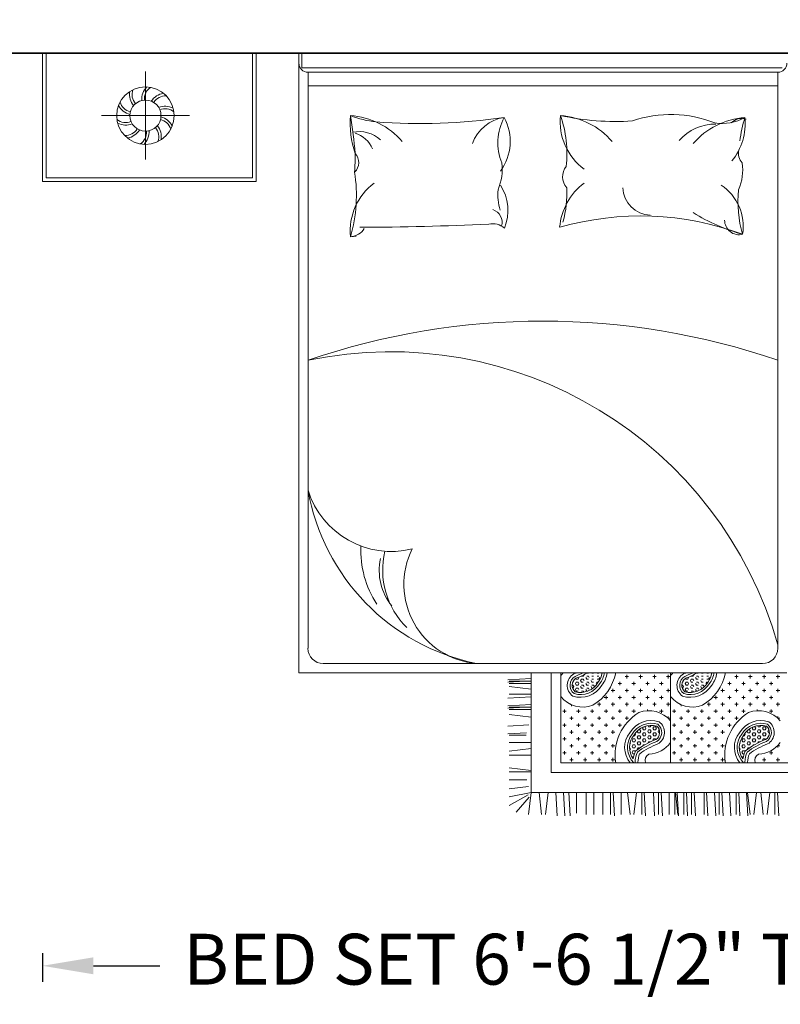
# Model space of a CAD drawing. Units: inches. Extents: x -638 to 186, y -762 to 59.
# Tile 23 of 31: x -125 to -66, y -126 to -48. Entities that reach past the tile are written whole.
import ezdxf

# ---------------------------------------------------------------- set-up
doc = ezdxf.new("R2010")
doc.units = ezdxf.units.IN
for name, color, linetype, lineweight in [('A-ANNO-DIMS', 2, 'Continuous', 18), ('furn', 8, 'Continuous', 13), ('wall', 7, 'Continuous', 35)]:
    doc.layers.add(name, color=color, linetype=linetype, lineweight=lineweight)
doc.styles.get("Standard").update_dxf_attribs({"font": 'arial.ttf'})
doc.dimstyles.new('ISO-25', dxfattribs={"dimtxt": 4, "dimasz": 4, "dimexe": 1.25, "dimexo": 0.625, "dimtad": 0, "dimlunit": 4, "dimtxsty": 'Standard', "dimcen": 2.5, "dimclrt": 256, "dimadec": 0, "dimazin": 0, "dimtfac": 1, "dimtmove": 0, "dimatfit": 3, "dimfxl": 1, "dimfxlon": 1, "dimarcsym": 0})

# ---------------------------------------------------------------- blocks, each defined once
blk = doc.blocks.new('BED-DOUBLE-WITH-NIGHTSTANDS')
for p, q in [((0, 59.951), (78.699, 59.951)), ((0, 49.874), (0, 59.951)), ((0.288, 50.162), (0.288, 59.951)), ((16.508, 59.951), (16.508, 50.162)), ((16.796, 59.951), (16.796, 49.874)), ((20.158, 59.951), (20.158, 11.244)), ((20.398, 58.826), (20.398, 59.951)), ((8.091, 51.596), (8.091, 58.516)), ((58.161, 58.826), (20.398, 58.826)), ((20.878, 58.468), (57.828, 58.468)), ((20.878, 58.468), (20.878, 13.164)), ((57.828, 13.164), (57.828, 58.468)), ((57.828, 57.404), (20.878, 57.404)), ((4.631, 55.056), (11.551, 55.056)), ((16.796, 49.874), (0, 49.874)), ((16.508, 50.162), (0.288, 50.162)), ((22.077, 11.964), (56.628, 11.964)), ((20.158, 11.244), (58.548, 11.244)), ((38.435, 1.829), (38.435, 11.244)), ((39.99, 3.384), (39.99, 11.244)), ((40.767, 4.161), (40.767, 11.244)), ((42.184, 10.861), (42.116, 10.743)), ((42.164, 10.895), (42.184, 10.861)), ((42.381, 10.99), (42.388, 10.979)), ((42.524, 10.979), (42.388, 10.979)), ((42.588, 11.09), (42.524, 10.979)), ((42.728, 10.861), (42.796, 10.743)), ((42.932, 10.979), (42.796, 10.979)), ((42.932, 11.215), (42.819, 11.215)), ((42.932, 10.979), (43, 10.861)), ((43.34, 11.215), (43.204, 11.215)), ((43.34, 10.979), (43.204, 10.979)), ((43.748, 11.215), (43.612, 11.215)), ((43.748, 10.979), (43.612, 10.979)), ((43.816, 10.861), (43.748, 10.743)), ((44.002, 11.184), (43.952, 11.097)), ((45.812, 10.936), (46.084, 10.936)), ((45.948, 10.8), (45.948, 11.072)), ((46.9, 10.936), (47.172, 10.936)), ((47.036, 10.8), (47.036, 11.072)), ((47.989, 10.936), (48.261, 10.936)), ((48.125, 10.8), (48.125, 11.072)), ((49.077, 10.936), (49.349, 10.936)), ((49.213, 10.8), (49.213, 11.072)), ((49.395, 11.244), (49.395, 4.161)), ((50.811, 10.861), (50.743, 10.743)), ((50.792, 10.895), (50.811, 10.861)), ((51.009, 10.99), (51.015, 10.979)), ((51.151, 10.979), (51.015, 10.979)), ((51.216, 11.09), (51.151, 10.979)), ((51.355, 10.861), (51.424, 10.743)), ((51.56, 10.979), (51.424, 10.979)), ((51.56, 11.215), (51.447, 11.215)), ((51.56, 10.979), (51.628, 10.861)), ((51.968, 11.215), (51.832, 11.215)), ((51.968, 10.979), (51.832, 10.979)), ((52.376, 11.215), (52.24, 11.215)), ((52.376, 10.979), (52.24, 10.979)), ((52.444, 10.861), (52.376, 10.743)), ((52.63, 11.184), (52.58, 11.097)), ((54.44, 10.936), (54.712, 10.936)), ((54.576, 10.8), (54.576, 11.072)), ((55.528, 10.936), (55.8, 10.936)), ((55.664, 10.8), (55.664, 11.072)), ((56.616, 10.936), (56.888, 10.936)), ((56.752, 10.8), (56.752, 11.072)), ((57.705, 10.936), (57.977, 10.936)), ((57.841, 10.8), (57.841, 11.072)), ((38.435, 10.789), (36.606, 10.687)), ((38.435, 10.606), (36.606, 10.504)), ((38.435, 10.585), (36.707, 10.585)), ((38.435, 10.402), (36.707, 10.402)), ((38.435, 9.957), (36.707, 10.161)), ((41.708, 10.272), (41.649, 10.272)), ((41.708, 10.508), (41.699, 10.508)), ((41.776, 10.625), (41.708, 10.508)), ((41.708, 10.272), (41.776, 10.154)), ((41.776, 10.154), (41.708, 10.036)), ((41.77, 10.636), (41.776, 10.625)), ((41.98, 10.508), (41.912, 10.39)), ((41.912, 10.39), (41.98, 10.272)), ((41.943, 10.806), (41.98, 10.743)), ((42.116, 10.743), (41.98, 10.743)), ((42.116, 10.508), (41.98, 10.508)), ((42.116, 10.272), (41.98, 10.272)), ((42.116, 10.508), (42.184, 10.39)), ((42.184, 10.39), (42.116, 10.272)), ((42.388, 10.743), (42.32, 10.625)), ((42.32, 10.625), (42.388, 10.508)), ((42.32, 10.154), (42.388, 10.036)), ((42.524, 10.743), (42.388, 10.743)), ((42.524, 10.508), (42.388, 10.508)), ((42.524, 10.272), (42.388, 10.272)), ((42.524, 10.743), (42.592, 10.625)), ((42.524, 10.272), (42.592, 10.154)), ((42.728, 10.39), (42.796, 10.272)), ((42.932, 10.743), (42.796, 10.743)), ((42.932, 10.508), (42.796, 10.508)), ((42.932, 10.272), (42.796, 10.272)), ((42.932, 10.508), (43, 10.39)), ((43.136, 10.625), (43.204, 10.508)), ((43.136, 10.154), (43.204, 10.036)), ((43.34, 10.743), (43.204, 10.743)), ((43.34, 10.508), (43.204, 10.508)), ((43.34, 10.272), (43.204, 10.272)), ((43.34, 10.272), (43.408, 10.154)), ((43.408, 10.154), (43.381, 10.108)), ((43.612, 10.508), (43.544, 10.39)), ((43.748, 10.743), (43.612, 10.743)), ((43.703, 10.508), (43.612, 10.508)), ((45.268, 10.392), (45.54, 10.392)), ((45.404, 10.256), (45.404, 10.528)), ((46.356, 10.392), (46.628, 10.392)), ((46.492, 10.256), (46.492, 10.528)), ((47.445, 10.392), (47.717, 10.392)), ((47.581, 10.256), (47.581, 10.528)), ((48.533, 10.392), (48.805, 10.392)), ((48.669, 10.256), (48.669, 10.528)), ((50.335, 10.272), (50.277, 10.272)), ((50.335, 10.508), (50.327, 10.508)), ((50.403, 10.625), (50.335, 10.508)), ((50.335, 10.272), (50.403, 10.154)), ((50.403, 10.154), (50.335, 10.036)), ((50.397, 10.636), (50.403, 10.625)), ((50.607, 10.508), (50.539, 10.39)), ((50.539, 10.39), (50.607, 10.272)), ((50.571, 10.806), (50.607, 10.743)), ((50.743, 10.743), (50.607, 10.743)), ((50.743, 10.508), (50.607, 10.508)), ((50.743, 10.272), (50.607, 10.272)), ((50.743, 10.508), (50.811, 10.39)), ((50.811, 10.39), (50.743, 10.272)), ((51.015, 10.743), (50.947, 10.625)), ((50.947, 10.625), (51.015, 10.508)), ((50.947, 10.154), (51.015, 10.036)), ((51.151, 10.743), (51.015, 10.743)), ((51.151, 10.508), (51.015, 10.508)), ((51.151, 10.272), (51.015, 10.272)), ((51.151, 10.743), (51.219, 10.625)), ((51.151, 10.272), (51.219, 10.154)), ((51.355, 10.39), (51.424, 10.272)), ((51.56, 10.743), (51.424, 10.743)), ((51.56, 10.508), (51.424, 10.508)), ((51.56, 10.272), (51.424, 10.272)), ((51.56, 10.508), (51.628, 10.39)), ((51.764, 10.625), (51.832, 10.508)), ((51.764, 10.154), (51.832, 10.036)), ((51.968, 10.743), (51.832, 10.743)), ((51.968, 10.508), (51.832, 10.508)), ((51.968, 10.272), (51.832, 10.272)), ((51.968, 10.272), (52.036, 10.154)), ((52.036, 10.154), (52.009, 10.108)), ((52.24, 10.508), (52.172, 10.39)), ((52.376, 10.743), (52.24, 10.743)), ((52.33, 10.508), (52.24, 10.508)), ((53.896, 10.392), (54.168, 10.392)), ((54.032, 10.256), (54.032, 10.528)), ((54.984, 10.392), (55.256, 10.392)), ((55.12, 10.256), (55.12, 10.528)), ((56.072, 10.392), (56.344, 10.392)), ((56.208, 10.256), (56.208, 10.528)), ((57.161, 10.392), (57.433, 10.392)), ((57.297, 10.256), (57.297, 10.528)), ((38.435, 9.347), (36.606, 9.245)), ((38.435, 9.55), (36.707, 9.55)), ((41.708, 10.036), (41.685, 10.036)), ((41.98, 10.036), (41.912, 9.919)), ((41.912, 9.919), (41.98, 9.801)), ((42.116, 10.036), (41.98, 10.036)), ((42.116, 9.801), (41.98, 9.801)), ((42.116, 10.036), (42.184, 9.919)), ((42.524, 10.036), (42.388, 10.036)), ((42.524, 9.801), (42.388, 9.801)), ((42.524, 9.801), (42.574, 9.713)), ((42.728, 9.919), (42.796, 9.801)), ((42.932, 10.036), (42.796, 10.036)), ((42.888, 9.801), (42.796, 9.801)), ((42.932, 10.036), (43, 9.919)), ((43.297, 10.036), (43.204, 10.036)), ((44.18, 9.303), (44.452, 9.303)), ((44.316, 9.167), (44.316, 9.439)), ((44.724, 9.847), (44.996, 9.847)), ((44.86, 9.711), (44.86, 9.983)), ((45.268, 9.303), (45.54, 9.303)), ((45.404, 9.167), (45.404, 9.439)), ((45.812, 9.847), (46.084, 9.847)), ((45.948, 9.711), (45.948, 9.983)), ((46.356, 9.303), (46.628, 9.303)), ((46.492, 9.167), (46.492, 9.439)), ((46.9, 9.847), (47.172, 9.847)), ((47.036, 9.711), (47.036, 9.983)), ((47.445, 9.303), (47.717, 9.303)), ((47.581, 9.167), (47.581, 9.439)), ((47.989, 9.847), (48.261, 9.847)), ((48.125, 9.711), (48.125, 9.983)), ((48.533, 9.303), (48.805, 9.303)), ((48.669, 9.167), (48.669, 9.439)), ((49.077, 9.847), (49.349, 9.847)), ((49.213, 9.711), (49.213, 9.983)), ((50.335, 10.036), (50.313, 10.036)), ((50.607, 10.036), (50.539, 9.919)), ((50.539, 9.919), (50.607, 9.801)), ((50.743, 10.036), (50.607, 10.036)), ((50.743, 9.801), (50.607, 9.801)), ((50.743, 10.036), (50.811, 9.919)), ((51.151, 10.036), (51.015, 10.036)), ((51.151, 9.801), (51.015, 9.801)), ((51.151, 9.801), (51.202, 9.713)), ((51.355, 9.919), (51.424, 9.801)), ((51.56, 10.036), (51.424, 10.036)), ((51.516, 9.801), (51.424, 9.801)), ((51.56, 10.036), (51.628, 9.919)), ((51.925, 10.036), (51.832, 10.036)), ((52.807, 9.303), (53.079, 9.303)), ((52.943, 9.167), (52.943, 9.439)), ((53.351, 9.847), (53.623, 9.847)), ((53.487, 9.711), (53.487, 9.983)), ((53.896, 9.303), (54.168, 9.303)), ((54.032, 9.167), (54.032, 9.439)), ((54.44, 9.847), (54.712, 9.847)), ((54.576, 9.711), (54.576, 9.983)), ((54.984, 9.303), (55.256, 9.303)), ((55.12, 9.167), (55.12, 9.439)), ((55.528, 9.847), (55.8, 9.847)), ((55.664, 9.711), (55.664, 9.983)), ((56.072, 9.303), (56.344, 9.303)), ((56.208, 9.167), (56.208, 9.439)), ((56.616, 9.847), (56.888, 9.847)), ((56.752, 9.711), (56.752, 9.983)), ((57.161, 9.303), (57.433, 9.303)), ((57.297, 9.167), (57.297, 9.439)), ((57.705, 9.847), (57.977, 9.847)), ((57.841, 9.711), (57.841, 9.983)), ((38.435, 8.736), (36.606, 8.634)), ((38.435, 8.553), (36.606, 8.451)), ((38.435, 8.532), (36.707, 8.532)), ((41.459, 8.759), (41.528, 8.759)), ((41.595, 8.623), (41.595, 8.728)), ((43.635, 8.759), (43.907, 8.759)), ((43.771, 8.623), (43.771, 8.895)), ((44.724, 8.759), (44.996, 8.759)), ((44.86, 8.623), (44.86, 8.895)), ((45.812, 8.759), (46.084, 8.759)), ((45.948, 8.623), (45.948, 8.895)), ((46.9, 8.759), (47.172, 8.759)), ((47.036, 8.623), (47.036, 8.895)), ((47.989, 8.759), (48.261, 8.759)), ((48.125, 8.623), (48.125, 8.895)), ((49.077, 8.759), (49.349, 8.759)), ((49.213, 8.623), (49.213, 8.895)), ((50.086, 8.759), (50.155, 8.759)), ((50.222, 8.623), (50.222, 8.728)), ((52.263, 8.759), (52.535, 8.759)), ((52.399, 8.623), (52.399, 8.895)), ((53.351, 8.759), (53.623, 8.759)), ((53.487, 8.623), (53.487, 8.895)), ((54.44, 8.759), (54.712, 8.759)), ((54.576, 8.623), (54.576, 8.895)), ((55.528, 8.759), (55.8, 8.759)), ((55.664, 8.623), (55.664, 8.895)), ((56.616, 8.759), (56.888, 8.759)), ((56.752, 8.623), (56.752, 8.895)), ((57.705, 8.759), (57.977, 8.759)), ((57.841, 8.623), (57.841, 8.895)), ((38.435, 8.349), (36.707, 8.349)), ((38.435, 7.757), (36.707, 7.961)), ((40.914, 8.215), (41.187, 8.215)), ((41.051, 8.079), (41.051, 8.351)), ((41.595, 7.535), (41.595, 7.807)), ((42.003, 8.215), (42.275, 8.215)), ((42.139, 8.079), (42.139, 8.351)), ((42.683, 7.535), (42.683, 7.807)), ((43.091, 8.215), (43.363, 8.215)), ((43.227, 8.079), (43.227, 8.351)), ((43.771, 7.535), (43.771, 7.807)), ((44.18, 8.215), (44.452, 8.215)), ((44.316, 8.079), (44.316, 8.351)), ((44.86, 7.535), (44.86, 7.807)), ((45.268, 8.215), (45.54, 8.215)), ((45.404, 8.079), (45.404, 8.351)), ((45.948, 7.535), (45.948, 7.807)), ((46.356, 8.215), (46.628, 8.215)), ((46.492, 8.079), (46.492, 8.351)), ((47.581, 8.253), (47.581, 8.351)), ((48.533, 8.215), (48.805, 8.215)), ((48.669, 8.079), (48.669, 8.351)), ((49.213, 7.653), (49.213, 7.807)), ((49.542, 8.215), (49.814, 8.215)), ((49.678, 8.079), (49.678, 8.351)), ((50.222, 7.535), (50.222, 7.807)), ((50.63, 8.215), (50.903, 8.215)), ((50.767, 8.079), (50.767, 8.351)), ((51.311, 7.535), (51.311, 7.807)), ((51.719, 8.215), (51.991, 8.215)), ((51.855, 8.079), (51.855, 8.351)), ((52.399, 7.535), (52.399, 7.807)), ((52.807, 8.215), (53.079, 8.215)), ((52.943, 8.079), (52.943, 8.351)), ((53.487, 7.535), (53.487, 7.807)), ((53.896, 8.215), (54.168, 8.215)), ((54.032, 8.079), (54.032, 8.351)), ((54.576, 7.535), (54.576, 7.807)), ((54.984, 8.215), (55.256, 8.215)), ((55.12, 8.079), (55.12, 8.351)), ((56.208, 8.253), (56.208, 8.351)), ((57.161, 8.215), (57.433, 8.215)), ((57.297, 8.079), (57.297, 8.351)), ((57.841, 7.653), (57.841, 7.807)), ((38.233, 7.135), (36.606, 7.044)), ((40.914, 7.127), (41.187, 7.127)), ((41.051, 6.99), (41.051, 7.263)), ((41.459, 7.671), (41.731, 7.671)), ((42.003, 7.127), (42.275, 7.127)), ((42.139, 6.99), (42.139, 7.263)), ((42.547, 7.671), (42.819, 7.671)), ((43.091, 7.127), (43.363, 7.127)), ((43.227, 6.99), (43.227, 7.263)), ((43.635, 7.671), (43.907, 7.671)), ((44.18, 7.127), (44.452, 7.127)), ((44.316, 6.99), (44.316, 7.263)), ((44.724, 7.671), (44.996, 7.671)), ((45.268, 7.127), (45.54, 7.127)), ((45.404, 6.99), (45.404, 7.263)), ((45.812, 7.671), (46.084, 7.671)), ((47.185, 6.877), (47.239, 6.971)), ((47.297, 6.995), (47.389, 6.995)), ((47.457, 6.877), (47.389, 6.995)), ((47.661, 6.995), (47.611, 7.082)), ((47.661, 6.995), (47.797, 6.995)), ((47.797, 6.995), (47.861, 7.105)), ((48.001, 6.877), (48.069, 6.995)), ((48.069, 6.995), (48.205, 6.995)), ((48.273, 6.877), (48.205, 6.995)), ((49.195, 7.671), (49.349, 7.671)), ((49.542, 7.127), (49.814, 7.127)), ((49.678, 6.99), (49.678, 7.263)), ((50.086, 7.671), (50.358, 7.671)), ((50.63, 7.127), (50.903, 7.127)), ((50.767, 6.99), (50.767, 7.263)), ((51.175, 7.671), (51.447, 7.671)), ((51.719, 7.127), (51.991, 7.127)), ((51.855, 6.99), (51.855, 7.263)), ((52.263, 7.671), (52.535, 7.671)), ((52.807, 7.127), (53.079, 7.127)), ((52.943, 6.99), (52.943, 7.263)), ((53.351, 7.671), (53.623, 7.671)), ((53.896, 7.127), (54.168, 7.127)), ((54.032, 6.99), (54.032, 7.263)), ((54.44, 7.671), (54.712, 7.671)), ((55.813, 6.877), (55.867, 6.971)), ((55.924, 6.995), (56.017, 6.995)), ((56.085, 6.877), (56.017, 6.995)), ((56.289, 6.995), (56.238, 7.082)), ((56.289, 6.995), (56.425, 6.995)), ((56.425, 6.995), (56.488, 7.105)), ((56.629, 6.877), (56.697, 6.995)), ((56.697, 6.995), (56.833, 6.995)), ((56.901, 6.877), (56.833, 6.995)), ((57.822, 7.671), (57.977, 7.671)), ((38.06, 6.514), (36.606, 6.433)), ((38.024, 6.332), (36.707, 6.332)), ((41.459, 6.582), (41.731, 6.582)), ((41.595, 6.446), (41.595, 6.718)), ((42.547, 6.582), (42.819, 6.582)), ((42.683, 6.446), (42.683, 6.718)), ((43.635, 6.582), (43.907, 6.582)), ((43.771, 6.446), (43.771, 6.718)), ((44.724, 6.582), (44.996, 6.582)), ((44.86, 6.446), (44.86, 6.718)), ((46.482, 6.288), (46.573, 6.288)), ((46.573, 6.288), (46.641, 6.406)), ((46.641, 6.406), (46.605, 6.469)), ((46.777, 6.642), (46.803, 6.688)), ((46.845, 6.524), (46.777, 6.642)), ((46.777, 6.17), (46.845, 6.288)), ((46.845, 6.524), (46.981, 6.524)), ((46.845, 6.288), (46.981, 6.288)), ((46.888, 6.76), (46.981, 6.76)), ((47.049, 6.642), (46.981, 6.76)), ((46.981, 6.524), (47.049, 6.642)), ((47.049, 6.17), (46.981, 6.288)), ((47.253, 6.76), (47.185, 6.877)), ((47.185, 6.406), (47.253, 6.524)), ((47.253, 6.288), (47.185, 6.406)), ((47.253, 6.76), (47.389, 6.76)), ((47.253, 6.524), (47.389, 6.524)), ((47.253, 6.288), (47.389, 6.288)), ((47.389, 6.76), (47.457, 6.877)), ((47.457, 6.406), (47.389, 6.524)), ((47.389, 6.288), (47.457, 6.406)), ((47.593, 6.642), (47.661, 6.76)), ((47.661, 6.524), (47.593, 6.642)), ((47.593, 6.17), (47.661, 6.288)), ((47.661, 6.76), (47.797, 6.76)), ((47.661, 6.524), (47.797, 6.524)), ((47.661, 6.288), (47.797, 6.288)), ((47.865, 6.642), (47.797, 6.76)), ((47.797, 6.524), (47.865, 6.642)), ((47.865, 6.17), (47.797, 6.288)), ((48.069, 6.76), (48.001, 6.877)), ((48.001, 6.406), (48.069, 6.524)), ((48.069, 6.288), (48.001, 6.406)), ((48.069, 6.76), (48.205, 6.76)), ((48.069, 6.524), (48.205, 6.524)), ((48.069, 6.288), (48.205, 6.288)), ((48.205, 6.76), (48.273, 6.877)), ((48.273, 6.406), (48.205, 6.524)), ((48.205, 6.288), (48.273, 6.406)), ((48.409, 6.642), (48.477, 6.76)), ((48.477, 6.524), (48.409, 6.642)), ((48.409, 6.17), (48.477, 6.288)), ((48.477, 6.76), (48.5, 6.76)), ((48.477, 6.524), (48.536, 6.524)), ((48.477, 6.288), (48.486, 6.288)), ((50.086, 6.582), (50.358, 6.582)), ((50.222, 6.446), (50.222, 6.718)), ((51.175, 6.582), (51.447, 6.582)), ((51.311, 6.446), (51.311, 6.718)), ((52.263, 6.582), (52.535, 6.582)), ((52.399, 6.446), (52.399, 6.718)), ((53.351, 6.582), (53.623, 6.582)), ((53.487, 6.446), (53.487, 6.718)), ((55.11, 6.288), (55.201, 6.288)), ((55.201, 6.288), (55.269, 6.406)), ((55.269, 6.406), (55.232, 6.469)), ((55.405, 6.642), (55.431, 6.688)), ((55.473, 6.524), (55.405, 6.642)), ((55.405, 6.17), (55.473, 6.288)), ((55.473, 6.524), (55.609, 6.524)), ((55.473, 6.288), (55.609, 6.288)), ((55.515, 6.76), (55.609, 6.76)), ((55.677, 6.642), (55.609, 6.76)), ((55.609, 6.524), (55.677, 6.642)), ((55.677, 6.17), (55.609, 6.288)), ((55.881, 6.76), (55.813, 6.877)), ((55.813, 6.406), (55.881, 6.524)), ((55.881, 6.288), (55.813, 6.406)), ((55.881, 6.76), (56.017, 6.76)), ((55.881, 6.524), (56.017, 6.524)), ((55.881, 6.288), (56.017, 6.288)), ((56.017, 6.76), (56.085, 6.877)), ((56.085, 6.406), (56.017, 6.524)), ((56.017, 6.288), (56.085, 6.406)), ((56.221, 6.642), (56.289, 6.76)), ((56.289, 6.524), (56.221, 6.642)), ((56.221, 6.17), (56.289, 6.288)), ((56.289, 6.76), (56.425, 6.76)), ((56.289, 6.524), (56.425, 6.524)), ((56.289, 6.288), (56.425, 6.288)), ((56.493, 6.642), (56.425, 6.76)), ((56.425, 6.524), (56.493, 6.642)), ((56.493, 6.17), (56.425, 6.288)), ((56.697, 6.76), (56.629, 6.877)), ((56.629, 6.406), (56.697, 6.524)), ((56.697, 6.288), (56.629, 6.406)), ((56.697, 6.76), (56.833, 6.76)), ((56.697, 6.524), (56.833, 6.524)), ((56.697, 6.288), (56.833, 6.288)), ((56.833, 6.76), (56.901, 6.877)), ((56.901, 6.406), (56.833, 6.524)), ((56.833, 6.288), (56.901, 6.406)), ((57.037, 6.642), (57.105, 6.76)), ((57.105, 6.524), (57.037, 6.642)), ((57.037, 6.17), (57.105, 6.288)), ((57.105, 6.76), (57.128, 6.76)), ((57.105, 6.524), (57.164, 6.524)), ((57.105, 6.288), (57.113, 6.288)), ((38.435, 5.764), (36.71, 5.764)), ((40.914, 6.038), (41.187, 6.038)), ((41.051, 5.902), (41.051, 6.174)), ((41.459, 5.494), (41.731, 5.494)), ((41.595, 5.358), (41.595, 5.63)), ((42.003, 6.038), (42.275, 6.038)), ((42.139, 5.902), (42.139, 6.174)), ((42.547, 5.494), (42.819, 5.494)), ((42.683, 5.358), (42.683, 5.63)), ((43.091, 6.038), (43.363, 6.038)), ((43.227, 5.902), (43.227, 6.174)), ((43.635, 5.494), (43.907, 5.494)), ((43.771, 5.358), (43.771, 5.63)), ((44.18, 6.038), (44.452, 6.038)), ((44.316, 5.902), (44.316, 6.174)), ((44.724, 5.494), (44.996, 5.494)), ((44.86, 5.358), (44.86, 5.63)), ((46.183, 5.612), (46.233, 5.699)), ((46.233, 5.699), (46.21, 5.739)), ((46.369, 5.935), (46.437, 6.053)), ((46.437, 5.817), (46.369, 5.935)), ((46.369, 5.464), (46.437, 5.581)), ((46.437, 5.346), (46.369, 5.464)), ((46.437, 6.053), (46.573, 6.053)), ((46.437, 5.817), (46.573, 5.817)), ((46.437, 5.581), (46.573, 5.581)), ((46.641, 5.935), (46.573, 6.053)), ((46.573, 5.817), (46.641, 5.935)), ((46.641, 5.464), (46.573, 5.581)), ((46.573, 5.346), (46.641, 5.464)), ((46.845, 6.053), (46.777, 6.17)), ((46.777, 5.699), (46.845, 5.817)), ((46.845, 5.581), (46.777, 5.699)), ((46.845, 6.053), (46.981, 6.053)), ((46.845, 5.817), (46.981, 5.817)), ((46.845, 5.581), (46.981, 5.581)), ((46.981, 6.053), (47.049, 6.17)), ((47.049, 5.699), (46.981, 5.817)), ((46.981, 5.581), (47.049, 5.699)), ((47.185, 5.935), (47.253, 6.053)), ((47.253, 5.817), (47.185, 5.935)), ((47.195, 5.481), (47.253, 5.581)), ((47.253, 6.053), (47.389, 6.053)), ((47.253, 5.817), (47.389, 5.817)), ((47.253, 5.581), (47.365, 5.581)), ((47.457, 5.935), (47.389, 6.053)), ((47.389, 5.817), (47.457, 5.935)), ((47.661, 6.053), (47.593, 6.17)), ((47.597, 5.706), (47.661, 5.817)), ((47.661, 6.053), (47.797, 6.053)), ((47.661, 5.817), (47.797, 5.817)), ((47.797, 6.053), (47.865, 6.17)), ((47.804, 5.806), (47.797, 5.817)), ((48.001, 5.935), (48.069, 6.053)), ((48.021, 5.901), (48.001, 5.935)), ((48.069, 6.053), (48.205, 6.053)), ((48.242, 5.99), (48.205, 6.053)), ((48.415, 6.16), (48.409, 6.17)), ((49.542, 6.038), (49.814, 6.038)), ((49.678, 5.902), (49.678, 6.174)), ((50.086, 5.494), (50.358, 5.494)), ((50.222, 5.358), (50.222, 5.63)), ((50.63, 6.038), (50.903, 6.038)), ((50.767, 5.902), (50.767, 6.174)), ((51.175, 5.494), (51.447, 5.494)), ((51.311, 5.358), (51.311, 5.63)), ((51.719, 6.038), (51.991, 6.038)), ((51.855, 5.902), (51.855, 6.174)), ((52.263, 5.494), (52.535, 5.494)), ((52.399, 5.358), (52.399, 5.63)), ((52.807, 6.038), (53.079, 6.038)), ((52.943, 5.902), (52.943, 6.174)), ((53.351, 5.494), (53.623, 5.494)), ((53.487, 5.358), (53.487, 5.63)), ((54.81, 5.612), (54.86, 5.699)), ((54.86, 5.699), (54.837, 5.739)), ((54.996, 5.935), (55.064, 6.053)), ((55.064, 5.817), (54.996, 5.935)), ((54.996, 5.464), (55.064, 5.581)), ((55.064, 5.346), (54.996, 5.464)), ((55.064, 6.053), (55.201, 6.053)), ((55.064, 5.817), (55.201, 5.817)), ((55.064, 5.581), (55.201, 5.581)), ((55.269, 5.935), (55.201, 6.053)), ((55.201, 5.817), (55.269, 5.935)), ((55.269, 5.464), (55.201, 5.581)), ((55.201, 5.346), (55.269, 5.464)), ((55.473, 6.053), (55.405, 6.17)), ((55.405, 5.699), (55.473, 5.817)), ((55.473, 5.581), (55.405, 5.699)), ((55.473, 6.053), (55.609, 6.053)), ((55.473, 5.817), (55.609, 5.817)), ((55.473, 5.581), (55.609, 5.581)), ((55.609, 6.053), (55.677, 6.17)), ((55.677, 5.699), (55.609, 5.817)), ((55.609, 5.581), (55.677, 5.699)), ((55.813, 5.935), (55.881, 6.053)), ((55.881, 5.817), (55.813, 5.935)), ((55.823, 5.481), (55.881, 5.581)), ((55.881, 6.053), (56.017, 6.053)), ((55.881, 5.817), (56.017, 5.817)), ((55.881, 5.581), (55.993, 5.581)), ((56.085, 5.935), (56.017, 6.053)), ((56.017, 5.817), (56.085, 5.935)), ((56.289, 6.053), (56.221, 6.17)), ((56.225, 5.706), (56.289, 5.817)), ((56.289, 6.053), (56.425, 6.053)), ((56.289, 5.817), (56.425, 5.817)), ((56.425, 6.053), (56.493, 6.17)), ((56.431, 5.806), (56.425, 5.817)), ((56.629, 5.935), (56.697, 6.053)), ((56.649, 5.901), (56.629, 5.935)), ((56.697, 6.053), (56.833, 6.053)), ((56.869, 5.99), (56.833, 6.053)), ((57.043, 6.16), (57.037, 6.17)), ((57.803, 5.494), (57.977, 5.494)), ((57.841, 5.358), (57.841, 5.533)), ((38.435, 5.274), (36.707, 5.069)), ((38.435, 4.769), (36.71, 4.769)), ((40.914, 4.95), (41.187, 4.95)), ((41.051, 4.814), (41.051, 5.086)), ((42.003, 4.95), (42.275, 4.95)), ((42.139, 4.814), (42.139, 5.086)), ((43.091, 4.95), (43.363, 4.95)), ((43.227, 4.814), (43.227, 5.086)), ((44.18, 4.95), (44.452, 4.95)), ((44.316, 4.814), (44.316, 5.086)), ((46.162, 5.346), (46.165, 5.346)), ((46.233, 5.228), (46.165, 5.346)), ((46.179, 5.135), (46.233, 5.228)), ((46.369, 4.992), (46.437, 5.11)), ((46.437, 4.874), (46.369, 4.992)), ((46.437, 5.346), (46.573, 5.346)), ((46.437, 5.11), (46.573, 5.11)), ((46.437, 4.874), (46.559, 4.874)), ((46.619, 5.03), (46.573, 5.11)), ((46.777, 5.228), (46.845, 5.346)), ((46.788, 5.209), (46.777, 5.228)), ((46.845, 5.346), (46.981, 5.346)), ((46.982, 5.344), (46.981, 5.346)), ((49.542, 4.95), (49.814, 4.95)), ((49.678, 4.814), (49.678, 5.086)), ((50.63, 4.95), (50.903, 4.95)), ((50.767, 4.814), (50.767, 5.086)), ((51.719, 4.95), (51.991, 4.95)), ((51.855, 4.814), (51.855, 5.086)), ((52.807, 4.95), (53.079, 4.95)), ((52.943, 4.814), (52.943, 5.086)), ((54.789, 5.346), (54.792, 5.346)), ((54.86, 5.228), (54.792, 5.346)), ((54.807, 5.135), (54.86, 5.228)), ((54.996, 4.992), (55.064, 5.11)), ((55.064, 4.874), (54.996, 4.992)), ((55.064, 5.346), (55.201, 5.346)), ((55.064, 5.11), (55.201, 5.11)), ((55.064, 4.874), (55.187, 4.874)), ((55.247, 5.03), (55.201, 5.11)), ((55.405, 5.228), (55.473, 5.346)), ((55.416, 5.209), (55.405, 5.228)), ((55.473, 5.346), (55.609, 5.346)), ((55.609, 5.344), (55.609, 5.346)), ((57.161, 4.95), (57.433, 4.95)), ((57.297, 4.814), (57.297, 5.086)), ((66.65, 4.161), (40.767, 4.161)), ((41.459, 4.406), (41.731, 4.406)), ((41.595, 4.27), (41.595, 4.542)), ((42.547, 4.406), (42.819, 4.406)), ((42.683, 4.27), (42.683, 4.542)), ((43.635, 4.406), (43.907, 4.406)), ((43.771, 4.27), (43.771, 4.542)), ((44.724, 4.406), (44.996, 4.406)), ((44.86, 4.27), (44.86, 4.542)), ((46.393, 4.563), (46.437, 4.639)), ((46.437, 4.639), (46.493, 4.639)), ((50.086, 4.406), (50.358, 4.406)), ((50.222, 4.27), (50.222, 4.542)), ((51.175, 4.406), (51.447, 4.406)), ((51.311, 4.27), (51.311, 4.542)), ((52.263, 4.406), (52.535, 4.406)), ((52.399, 4.27), (52.399, 4.542)), ((53.351, 4.406), (53.623, 4.406)), ((53.487, 4.27), (53.487, 4.542)), ((55.021, 4.563), (55.064, 4.639)), ((55.064, 4.639), (55.12, 4.639)), ((56.616, 4.406), (56.888, 4.406)), ((56.752, 4.27), (56.752, 4.542)), ((57.705, 4.406), (57.977, 4.406)), ((57.841, 4.27), (57.841, 4.542)), ((38.435, 3.565), (36.707, 3.769)), ((38.435, 3.446), (36.71, 3.446)), ((67.427, 3.384), (39.99, 3.384)), ((38.086, 2.81), (36.71, 2.81)), ((38.221, 2.295), (36.707, 2.115)), ((38.185, 1.631), (36.707, 0.792)), ((38.421, 1.829), (36.71, 1.486)), ((38.435, 1.829), (38.231, 0.102)), ((68.982, 1.829), (38.435, 1.829)), ((39.046, 1.815), (39.249, 0.102)), ((39.759, 1.829), (39.555, 0.102)), ((40.369, 1.829), (40.471, 0)), ((40.98, 1.829), (41.082, 0)), ((41.388, 1.829), (41.49, 0)), ((41.999, 1.829), (41.999, 0.203)), ((42.744, 1.829), (42.744, 0.102)), ((43.355, 1.829), (43.355, 0.102)), ((44.068, 1.829), (44.068, 0.102)), ((44.679, 1.829), (44.679, 0.102)), ((44.882, 1.829), (44.984, 0)), ((45.511, 1.815), (45.511, 0.105)), ((46.002, 1.815), (46.206, 0.102)), ((46.715, 1.829), (46.512, 0.102)), ((47.122, 1.829), (47.122, 0.102)), ((47.326, 1.829), (47.428, 0)), ((48.039, 1.829), (48.141, 0)), ((48.446, 1.829), (48.446, 0.102)), ((48.65, 1.829), (48.752, 0)), ((49.279, 1.815), (49.279, 0.105)), ((49.717, 1.829), (49.717, 0.102)), ((49.77, 1.815), (49.973, 0.102)), ((49.92, 1.829), (50.022, 0)), ((50.429, 1.829), (50.429, 0.102)), ((50.633, 1.829), (50.735, 0)), ((51.04, 1.829), (51.04, 0.102)), ((51.244, 1.829), (51.346, 0)), ((52.025, 1.829), (52.025, 0.102)), ((52.229, 1.829), (52.331, 0)), ((52.84, 1.829), (52.942, 0)), ((53.221, 1.829), (53.221, 0.102)), ((53.424, 1.829), (53.526, 0)), ((54.035, 1.829), (54.137, 0)), ((54.544, 1.829), (54.544, 0.102)), ((54.748, 1.829), (54.85, 0)), ((55.359, 1.829), (55.461, 0)), ((55.442, 1.815), (55.646, 0.102)), ((56.155, 1.829), (55.951, 0.102)), ((56.479, 1.815), (56.683, 0.102)), ((57.192, 1.829), (56.988, 0.102)), ((57.599, 1.829), (57.599, 0.102)), ((57.803, 1.829), (57.905, 0)), ((38.274, 1.47), (37.248, 0.275))]:
    blk.add_line(p, q)
for radius in [2.26, 1.225]:
    blk.add_circle((8.091, 55.056), radius)
for centre, radius, start, end in [((20.878, 59.188), 0.72, 180, 270), ((57.828, 59.188), 0.72, 270, 0), ((9.248, 56.308), 1.452, 136.17003, 182.48975), ((8.292, 56.749), 1.452, 172.17003, 218.48975), ((8.15, 56.718), 1.108, 160.30017, 220.53802), ((9.115, 56.366), 1.108, 124.30017, 184.53802), ((9.763, 55.389), 1.452, 100.17003, 146.48975), ((9.69, 55.514), 1.108, 88.30017, 148.53802), ((7.258, 56.544), 1.452, 208.17003, 254.48975), ((7.162, 56.435), 1.108, 196.30017, 256.53802), ((9.64, 54.343), 1.452, 64.17003, 110.48975), ((9.653, 54.487), 1.108, 52.30017, 112.53802), ((31.6, 54.462), 7.401, 175.30484, 198.69419), ((-14.535, 48.797), 39.263, 4.80985, 9.18918), ((26.929, 61.603), 7.073, 247.51785, 264.26696), ((23.812, 49.204), 5.878, 40.4189, 85.9871), ((45.371, 54.589), 4.662, 174.11002, 233.4289), ((45.094, 75.141), 20.542, 257.74383, 273.62843), ((40.322, 49.204), 5.878, 40.4189, 85.9871), ((32.161, 52.085), 9.076, 353.49469, 19.18669), ((49.42, 45.842), 9.304, 68.20259, 108.9817), ((6.529, 55.625), 1.108, 232.30017, 292.53802), ((6.543, 55.77), 1.452, 244.17003, 290.48975), ((7.891, 53.363), 1.452, 352.17003, 38.48975), ((9.021, 53.678), 1.108, 16.30017, 76.53802), ((8.925, 53.569), 1.452, 28.17003, 74.48975), ((29.668, 101.849), 47.41, 265.83211, 278.05982), ((36.728, 51.85), 3.086, 97.70317, 160.97754), ((40.051, 52.903), 4.24, 151.77364, 201.69827), ((32.811, 53.035), 3.973, 323.73888, 28.12687), ((52.894, 50.642), 3.752, 88.95772, 139.05179), ((55.647, 49.045), 5.878, 94.0129, 139.5811), ((53.423, 58.191), 3.75, 261.59582, 298.90918), ((54.987, 53.651), 1.175, 72.9226, 134.40089), ((50.598, 54.43), 4.662, 320.94042, 5.88999), ((67.137, 51.406), 12.406, 163.60457, 172.3273), ((6.493, 54.599), 1.108, 268.30017, 328.53802), ((6.419, 54.723), 1.452, 280.17003, 326.48975), ((7.067, 53.747), 1.108, 304.30017, 4.53802), ((6.934, 53.804), 1.452, 316.17003, 2.48975), ((8.033, 53.395), 1.108, 340.30017, 40.53802), ((24.909, 51.33), 2.472, 47.45091, 101.77931), ((23.874, 51.513), 2.284, 23.87557, 72.13833), ((23.796, 51.371), 1.071, 314.4736, 42.17134), ((-32.064, 53.187), 56.669, 357.39054, 358.88764), ((55.833, 52.089), 1.101, 165.35061, 223.26844), ((32.112, 50.806), 4.034, 337.01696, 7.53676), ((51.033, 50.806), 4.034, 337.01696, 7.53676), ((12.792, 48.807), 11.891, 344.0243, 8.70709), ((42.214, 50.25), 1.313, 142.08329, 220.902), ((28.862, 46.013), 4.662, 126.5711, 185.88998), ((32.952, 47.606), 3.653, 337.44667, 33.04781), ((45.546, 45.855), 4.894, 127.11975, 175.09005), ((51.147, 46.324), 3.96, 351.26213, 55.75721), ((40.21, 48.864), 4.4, 175.22328, 196.23004), ((33.322, 48.899), 7.916, 343.79543, 3.55541), ((47.91, 49.493), 2.28, 182.63002, 266.88402), ((63.68, 48.265), 8.986, 173.82958, 196.4356), ((35.105, 46.659), 1.047, 343.35206, 73.29947), ((59.196, 60.444), 15.291, 238.34989, 254.31375), ((24.019, 282.807), 236.536, 270.22759, 272.68343), ((35.378, 45.11), 1.447, 49.09906, 101.37023), ((47.026, 24.056), 23.109, 69.65065, 105.96307), ((54.788, 46.836), 1.147, 179.77267, 283.80184), ((24.141, 46.898), 1.366, 273.47085, 328.54118), ((23.812, 51.397), 5.878, 274.0129, 278.34166), ((39.353, -18.016), 56.914, 71.05766, 108.94234), ((27.358, 4.824), 31.662, 15.77081, 101.80991), ((37.529, 28.521), 16.903, 189.91062, 258.38345), ((27.435, 27.646), 6.865, 197.236, 283.86348), ((32.674, 20.841), 7.64, 177.22468, 213.41029), ((34.672, 18.19), 6.25, 153.48354, 264.97652), ((30.992, 19.307), 4.516, 168.35906, 218.53383), ((33.202, 19.362), 6.454, 167.11557, 225.10482), ((22.077, 13.164), 1.2, 180, 270), ((56.628, 13.164), 1.2, 270, 360), ((42.601, 9.717), 2.246, 137.14315, 144.73933), ((42.315, 10.253), 1.047, 120.34402, 234.01917), ((42.315, 10.253), 0.829, 121.62322, 231.69571), ((39.887, 16.395), 5.571, 289.92189, 292.41183), ((39.887, 16.395), 5.789, 290.13177, 297.16349), ((39.887, 16.395), 5.952, 290.29972, 300.08235), ((41.275, 12.01), 3.88, 301.11254, 348.61386), ((42.526, 11.434), 1.497, 320.65411, 352.72896), ((42.526, 11.434), 1.66, 321.11073, 353.44716), ((42.526, 11.434), 1.878, 321.59726, 354.2094), ((51.228, 9.717), 2.246, 137.14315, 144.73933), ((50.942, 10.253), 1.047, 120.34402, 234.01917), ((50.942, 10.253), 0.829, 121.62322, 231.69571), ((48.515, 16.395), 5.571, 289.92189, 292.41183), ((48.515, 16.395), 5.789, 290.13177, 297.16349), ((48.515, 16.395), 5.952, 290.29972, 300.08235), ((49.903, 12.01), 3.88, 301.11254, 348.61386), ((51.154, 11.434), 1.497, 320.65411, 352.72896), ((51.154, 11.434), 1.66, 321.11073, 353.44716), ((51.154, 11.434), 1.878, 321.59726, 354.2094), ((42.315, 10.253), 0.666, 122.94981, 229.099), ((42.307, 11.282), 1.972, 252.05502, 329.01896), ((42.307, 11.282), 1.754, 253.21886, 329.48085), ((42.307, 11.282), 1.591, 254.37381, 329.91174), ((50.942, 10.253), 0.666, 122.94981, 229.099), ((50.935, 11.282), 1.972, 252.05502, 329.01896), ((50.935, 11.282), 1.754, 253.21886, 329.48085), ((50.935, 11.282), 1.591, 254.37381, 329.91174), ((42.485, 10.742), 2.202, 218.7027, 291.15831), ((51.113, 10.742), 2.202, 218.7027, 291.15831), ((48.91, 4.786), 3.88, 121.11254, 189.2666), ((47.7, 6.054), 2.202, 39.66533, 111.15831), ((57.538, 4.786), 3.88, 121.11254, 189.2666), ((56.328, 6.054), 2.202, 39.66533, 111.15831), ((47.878, 5.514), 1.972, 72.05502, 149.01896), ((47.878, 5.514), 1.754, 73.21886, 149.48085), ((47.878, 5.514), 1.591, 74.37381, 149.91174), ((47.87, 6.543), 0.666, 302.94981, 49.099), ((47.87, 6.543), 0.829, 301.62322, 51.69571), ((47.87, 6.543), 1.047, 300.34402, 54.01917), ((56.505, 5.514), 1.972, 72.05502, 149.01896), ((56.505, 5.514), 1.754, 73.21886, 149.48085), ((56.505, 5.514), 1.591, 74.37381, 149.91174), ((56.498, 6.543), 0.666, 302.94981, 49.099), ((56.498, 6.543), 0.829, 301.62322, 51.69571), ((56.498, 6.543), 1.047, 300.34402, 54.01917), ((47.659, 5.362), 1.878, 141.59726, 219.76108), ((47.659, 5.362), 1.66, 141.11073, 226.3387), ((47.659, 5.362), 1.497, 140.65411, 216.833), ((56.286, 5.362), 1.878, 141.59726, 219.76108), ((56.286, 5.362), 1.66, 141.11073, 226.3387), ((56.286, 5.362), 1.497, 140.65411, 216.833), ((50.298, 0.401), 5.952, 110.29972, 127.73852), ((50.298, 0.401), 5.789, 110.13177, 127.34596), ((50.298, 0.401), 5.571, 109.92189, 126.76774), ((47.584, 7.079), 2.246, 272.46753, 323.71933), ((58.925, 0.401), 5.952, 110.29972, 127.73852), ((58.925, 0.401), 5.789, 110.13177, 127.34596), ((58.925, 0.401), 5.571, 109.92189, 126.76774), ((56.212, 7.079), 2.246, 272.46753, 323.71933), ((48.704, 4.14), 2.268, 154.70595, 171.7535), ((48.704, 4.14), 2.104, 155.76091, 178.03728), ((48.704, 4.14), 1.887, 157.40908, 178.03728), ((47.926, 4.355), 0.54, 117.00881, 201.04089), ((57.332, 4.14), 2.268, 154.70595, 171.7535), ((57.332, 4.14), 2.104, 155.76091, 178.03728), ((57.332, 4.14), 1.887, 157.40908, 178.03728), ((56.554, 4.355), 0.54, 117.00881, 201.04089)]:
    blk.add_arc(centre, radius, start, end)
blk = doc.blocks.new('*D27')
at = {"layer": 'A-ANNO-DIMS', "color": 0, "lineweight": -2, "transparency": 16777216}
for p, q in [((-123.625, -121.818), (-123.625, -124.068)), ((-44.925, -121.818), (-44.925, -124.068)), ((-119.625, -122.818), (-114.394, -122.818)), ((-48.925, -122.818), (-54.156, -122.818))]:
    blk.add_line(p, q, dxfattribs=at)
at = {"layer": 'A-ANNO-DIMS', "color": 0, "lineweight": 30, "transparency": 16777216}
for points in [[(-119.625, -122.151), (-119.625, -123.485), (-123.625, -122.818)], [(-48.925, -122.151), (-48.925, -123.485), (-44.925, -122.818)]]:
    blk.add_solid(points, dxfattribs=at)
at = {"layer": 'Defpoints', "color": 0, "lineweight": 30, "transparency": 16777216}
for p in [(-123.625, -111.013), (-44.925, -111.013), (-44.925, -122.818)]:
    blk.add_point(p, dxfattribs=at)
at = {"layer": 'A-ANNO-DIMS', "transparency": 16777216, "insert": (-84.275, -122.818), "char_height": 4, "attachment_point": 5}
blk.add_mtext('BED SET 6\'-6 1/2" TYP.', dxfattribs=at)
blk = doc.blocks.new('*D56')
at = {"layer": 'A-ANNO-DIMS', "color": 0, "lineweight": -2, "transparency": 16777216}
for p, q in [((-165.026, 52.017), (-165.026, 54.267)), ((-100.526, 52.017), (-100.526, 54.267)), ((-161.026, 53.017), (-143.378, 53.017)), ((-104.526, 53.017), (-122.174, 53.017))]:
    blk.add_line(p, q, dxfattribs=at)
at = {"layer": 'A-ANNO-DIMS', "color": 0, "lineweight": 30, "transparency": 16777216}
for points in [[(-161.026, 53.684), (-161.026, 52.35), (-165.026, 53.017)], [(-104.526, 53.684), (-104.526, 52.35), (-100.526, 53.017)]]:
    blk.add_solid(points, dxfattribs=at)
at = {"layer": 'Defpoints', "color": 0, "lineweight": 30, "transparency": 16777216}
for p in [(-100.526, 53.017), (-165.026, -408.033), (-100.526, -408.033)]:
    blk.add_point(p, dxfattribs=at)
at = {"layer": 'A-ANNO-DIMS', "transparency": 16777216, "insert": (-132.776, 53.017), "char_height": 4, "attachment_point": 5}
blk.add_mtext('5\'-4 1/2"', dxfattribs=at)

msp = doc.modelspace()

# ---------------------------------------------------------------- linework, layer by layer
at = {"layer": 'wall'}
msp.add_line((-160.526, -51.033), (1.474, -51.033), dxfattribs=at)
msp.add_line((-160.526, -51.033), (1.474, -51.033), dxfattribs=at)

# ---------------------------------------------------------------- block references
at = {"layer": 'furn'}
msp.add_blockref('BED-DOUBLE-WITH-NIGHTSTANDS', (-123.625, -111.013), dxfattribs=at)

# ---------------------------------------------------------------- dimensions: what is measured, and where the dimension line sits
at = {"layer": 'A-ANNO-DIMS'}
dim = msp.add_linear_dim(base=(-100.526, 53.017), p1=(-165.026, -408.033), p2=(-100.526, -408.033), dimstyle='ISO-25', override={"dimdec": 1, "dimlfac": 1, "dimrnd": 0, "dimzin": 1, "dimdsep": 46, "dimlunit": 4, "dimfrac": 2}, dxfattribs=at)
dim.commit()
dim.dimension.update_dxf_attribs({"geometry": '*D56', "text_midpoint": (-132.776, 53.017)})
dim = msp.add_linear_dim(base=(-44.925, -122.818), p1=(-123.625, -111.013), p2=(-44.925, -111.013), text='BED SET <> TYP.', dimstyle='ISO-25', override={"dimdec": 1, "dimlfac": 1, "dimrnd": 0, "dimzin": 1, "dimdsep": 46, "dimlunit": 4, "dimfrac": 2}, dxfattribs=at)
dim.commit()
dim.dimension.update_dxf_attribs({"geometry": '*D27', "text_midpoint": (-84.275, -122.818)})

doc.saveas('drawing.dxf')
